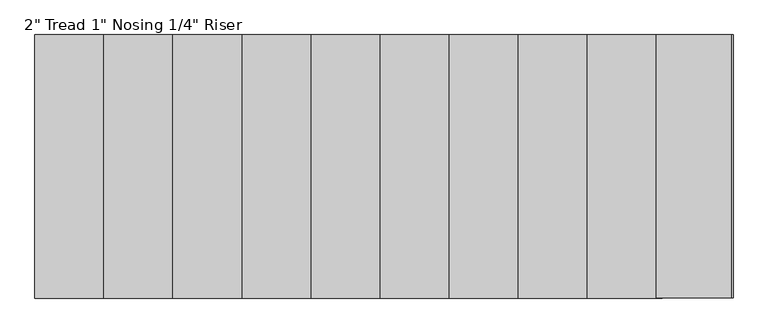
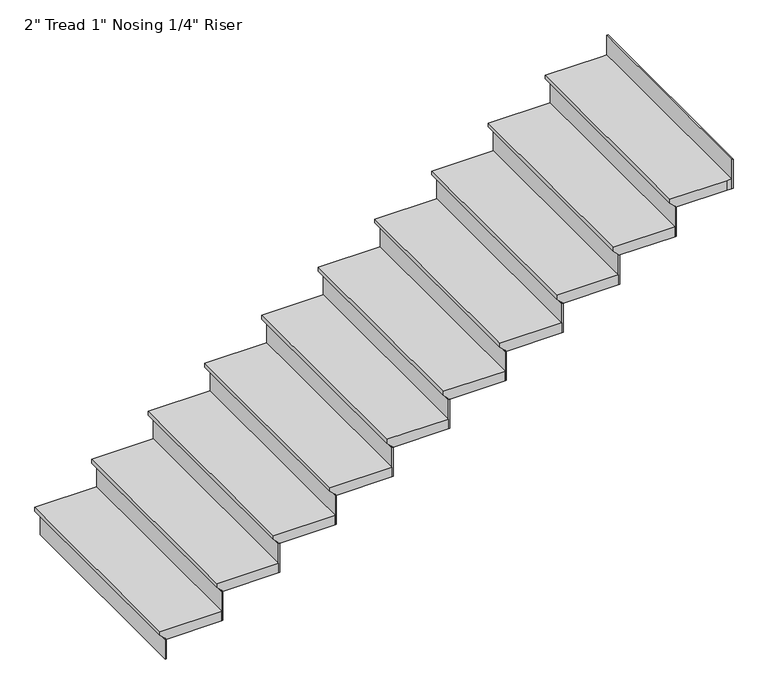
"""IFC4 building model written with IfcOpenShell, lengths in millimetres: stair flight geometry."""

from ifc_helpers import new_model, si_unit, origin, place, context, project, spatial, faceted_brep, source, transform, mapped, element, save


def stair_flight_b15b2b3c(model_context):
    return source(origin(), model_context, "Body", "Brep", [
        faceted_brep([(-459.26646, -1849.1834702, 6229.35), (-459.26646, -1849.1834702, 6248.4), (-459.26646, -782.3834702, 6248.4), (-459.26646, -782.3834702, 6229.35), (-433.86646, -1849.1834702, 6203.95), (-433.86646, -782.3834702, 6203.95), (-154.46646, -1849.1834702, 6248.4), (-154.46646, -782.3834702, 6248.4), (-433.86646, -782.3834702, 6197.6), (-154.46646, -782.3834702, 6197.6), (-154.46646, -1849.1834702, 6197.6), (-433.86646, -1849.1834702, 6197.6)], [[[0, 1, 2, 3]], [[4, 0, 3, 5]], [[2, 1, 6, 7]], [[8, 9, 10, 11]], [[2, 7, 9, 8, 5, 3]], [[8, 11, 4, 5]], [[6, 1, 0, 4, 11, 10]], [[7, 6, 10, 9]]]),
        faceted_brep([(-433.86646, -1849.1834702, 6197.6), (-433.86646, -1849.1834702, 6096.0), (-427.51646, -1849.1834702, 6096.0), (-427.51646, -1849.1834702, 6197.6), (-433.86646, -782.3834702, 6197.6), (-427.51646, -782.3834702, 6197.6), (-427.51646, -782.3834702, 6096.0), (-433.86646, -782.3834702, 6096.0)], [[[0, 1, 2, 3]], [[4, 5, 6, 7]], [[1, 0, 4, 7]], [[2, 1, 7, 6]], [[3, 2, 6, 5]], [[0, 3, 5, 4]]]),
        faceted_brep([(-154.46646, -1849.1834702, 6350.0), (-154.46646, -1849.1834702, 6197.6), (-148.11646, -1849.1834702, 6197.6), (-148.11646, -1849.1834702, 6350.0), (-154.46646, -782.3834702, 6350.0), (-148.11646, -782.3834702, 6350.0), (-148.11646, -782.3834702, 6197.6), (-154.46646, -782.3834702, 6197.6)], [[[0, 1, 2, 3]], [[4, 5, 6, 7]], [[1, 0, 4, 7]], [[2, 1, 7, 6]], [[3, 2, 6, 5]], [[0, 3, 5, 4]]]),
        faceted_brep([(-179.86646, -782.3834702, 6400.8), (-179.86646, -1849.1834702, 6400.8), (124.93354, -1849.1834702, 6400.8), (124.93354, -782.3834702, 6400.8), (-154.46646, -782.3834702, 6350.0), (124.93354, -782.3834702, 6350.0), (124.93354, -1849.1834702, 6350.0), (-154.46646, -1849.1834702, 6350.0), (-154.46646, -782.3834702, 6356.35), (-179.86646, -782.3834702, 6381.75), (-154.46646, -1849.1834702, 6356.35), (-179.86646, -1849.1834702, 6381.75)], [[[0, 1, 2, 3]], [[4, 5, 6, 7]], [[0, 3, 5, 4, 8, 9]], [[4, 7, 10, 8]], [[2, 1, 11, 10, 7, 6]], [[3, 2, 6, 5]], [[11, 1, 0, 9]], [[10, 11, 9, 8]]]),
        faceted_brep([(124.93354, -1849.1834702, 6502.4), (124.93354, -1849.1834702, 6350.0), (131.28354, -1849.1834702, 6350.0), (131.28354, -1849.1834702, 6502.4), (124.93354, -782.3834702, 6502.4), (131.28354, -782.3834702, 6502.4), (131.28354, -782.3834702, 6350.0), (124.93354, -782.3834702, 6350.0)], [[[0, 1, 2, 3]], [[4, 5, 6, 7]], [[1, 0, 4, 7]], [[2, 1, 7, 6]], [[3, 2, 6, 5]], [[0, 3, 5, 4]]]),
        faceted_brep([(99.53354, -782.3834702, 6553.2), (99.53354, -1849.1834702, 6553.2), (404.33354, -1849.1834702, 6553.2), (404.33354, -782.3834702, 6553.2), (124.93354, -782.3834702, 6502.4), (404.33354, -782.3834702, 6502.4), (404.33354, -1849.1834702, 6502.4), (124.93354, -1849.1834702, 6502.4), (124.93354, -782.3834702, 6508.75), (99.53354, -782.3834702, 6534.15), (124.93354, -1849.1834702, 6508.75), (99.53354, -1849.1834702, 6534.15)], [[[0, 1, 2, 3]], [[4, 5, 6, 7]], [[0, 3, 5, 4, 8, 9]], [[4, 7, 10, 8]], [[2, 1, 11, 10, 7, 6]], [[3, 2, 6, 5]], [[11, 1, 0, 9]], [[10, 11, 9, 8]]]),
        faceted_brep([(404.33354, -1849.1834702, 6654.8), (404.33354, -1849.1834702, 6502.4), (410.68354, -1849.1834702, 6502.4), (410.68354, -1849.1834702, 6654.8), (404.33354, -782.3834702, 6654.8), (410.68354, -782.3834702, 6654.8), (410.68354, -782.3834702, 6502.4), (404.33354, -782.3834702, 6502.4)], [[[0, 1, 2, 3]], [[4, 5, 6, 7]], [[1, 0, 4, 7]], [[2, 1, 7, 6]], [[3, 2, 6, 5]], [[0, 3, 5, 4]]]),
        faceted_brep([(378.93354, -782.3834702, 6705.6), (378.93354, -1849.1834702, 6705.6), (683.73354, -1849.1834702, 6705.6), (683.73354, -782.3834702, 6705.6), (404.33354, -782.3834702, 6654.8), (683.73354, -782.3834702, 6654.8), (683.73354, -1849.1834702, 6654.8), (404.33354, -1849.1834702, 6654.8), (404.33354, -782.3834702, 6661.15), (378.93354, -782.3834702, 6686.55), (404.33354, -1849.1834702, 6661.15), (378.93354, -1849.1834702, 6686.55)], [[[0, 1, 2, 3]], [[4, 5, 6, 7]], [[0, 3, 5, 4, 8, 9]], [[4, 7, 10, 8]], [[2, 1, 11, 10, 7, 6]], [[3, 2, 6, 5]], [[11, 1, 0, 9]], [[10, 11, 9, 8]]]),
        faceted_brep([(683.73354, -1849.1834702, 6807.2), (683.73354, -1849.1834702, 6654.8), (690.08354, -1849.1834702, 6654.8), (690.08354, -1849.1834702, 6807.2), (683.73354, -782.3834702, 6807.2), (690.08354, -782.3834702, 6807.2), (690.08354, -782.3834702, 6654.8), (683.73354, -782.3834702, 6654.8)], [[[0, 1, 2, 3]], [[4, 5, 6, 7]], [[1, 0, 4, 7]], [[2, 1, 7, 6]], [[3, 2, 6, 5]], [[0, 3, 5, 4]]]),
        faceted_brep([(658.33354, -782.3834702, 6858.0), (658.33354, -1849.1834702, 6858.0), (963.13354, -1849.1834702, 6858.0), (963.13354, -782.3834702, 6858.0), (683.73354, -782.3834702, 6807.2), (963.13354, -782.3834702, 6807.2), (963.13354, -1849.1834702, 6807.2), (683.73354, -1849.1834702, 6807.2), (683.73354, -782.3834702, 6813.55), (658.33354, -782.3834702, 6838.95), (683.73354, -1849.1834702, 6813.55), (658.33354, -1849.1834702, 6838.95)], [[[0, 1, 2, 3]], [[4, 5, 6, 7]], [[0, 3, 5, 4, 8, 9]], [[4, 7, 10, 8]], [[2, 1, 11, 10, 7, 6]], [[3, 2, 6, 5]], [[11, 1, 0, 9]], [[10, 11, 9, 8]]]),
        faceted_brep([(963.13354, -1849.1834702, 6959.6), (963.13354, -1849.1834702, 6807.2), (969.48354, -1849.1834702, 6807.2), (969.48354, -1849.1834702, 6959.6), (963.13354, -782.3834702, 6959.6), (969.48354, -782.3834702, 6959.6), (969.48354, -782.3834702, 6807.2), (963.13354, -782.3834702, 6807.2)], [[[0, 1, 2, 3]], [[4, 5, 6, 7]], [[1, 0, 4, 7]], [[2, 1, 7, 6]], [[3, 2, 6, 5]], [[0, 3, 5, 4]]]),
        faceted_brep([(937.73354, -782.3834702, 7010.4), (937.73354, -1849.1834702, 7010.4), (1242.53354, -1849.1834702, 7010.4), (1242.53354, -782.3834702, 7010.4), (963.13354, -782.3834702, 6959.6), (1242.53354, -782.3834702, 6959.6), (1242.53354, -1849.1834702, 6959.6), (963.13354, -1849.1834702, 6959.6), (963.13354, -782.3834702, 6965.95), (937.73354, -782.3834702, 6991.35), (963.13354, -1849.1834702, 6965.95), (937.73354, -1849.1834702, 6991.35)], [[[0, 1, 2, 3]], [[4, 5, 6, 7]], [[0, 3, 5, 4, 8, 9]], [[4, 7, 10, 8]], [[2, 1, 11, 10, 7, 6]], [[3, 2, 6, 5]], [[11, 1, 0, 9]], [[10, 11, 9, 8]]]),
        faceted_brep([(1242.53354, -1849.1834702, 7112.0), (1242.53354, -1849.1834702, 6959.6), (1248.88354, -1849.1834702, 6959.6), (1248.88354, -1849.1834702, 7112.0), (1242.53354, -782.3834702, 7112.0), (1248.88354, -782.3834702, 7112.0), (1248.88354, -782.3834702, 6959.6), (1242.53354, -782.3834702, 6959.6)], [[[0, 1, 2, 3]], [[4, 5, 6, 7]], [[1, 0, 4, 7]], [[2, 1, 7, 6]], [[3, 2, 6, 5]], [[0, 3, 5, 4]]]),
        faceted_brep([(1217.13354, -782.3834702, 7162.8), (1217.13354, -1849.1834702, 7162.8), (1521.93354, -1849.1834702, 7162.8), (1521.93354, -782.3834702, 7162.8), (1242.53354, -782.3834702, 7112.0), (1521.93354, -782.3834702, 7112.0), (1521.93354, -1849.1834702, 7112.0), (1242.53354, -1849.1834702, 7112.0), (1242.53354, -782.3834702, 7118.35), (1217.13354, -782.3834702, 7143.75), (1242.53354, -1849.1834702, 7118.35), (1217.13354, -1849.1834702, 7143.75)], [[[0, 1, 2, 3]], [[4, 5, 6, 7]], [[0, 3, 5, 4, 8, 9]], [[4, 7, 10, 8]], [[2, 1, 11, 10, 7, 6]], [[3, 2, 6, 5]], [[11, 1, 0, 9]], [[10, 11, 9, 8]]]),
        faceted_brep([(1521.93354, -1849.1834702, 7264.4), (1521.93354, -1849.1834702, 7112.0), (1528.28354, -1849.1834702, 7112.0), (1528.28354, -1849.1834702, 7264.4), (1521.93354, -782.3834702, 7264.4), (1528.28354, -782.3834702, 7264.4), (1528.28354, -782.3834702, 7112.0), (1521.93354, -782.3834702, 7112.0)], [[[0, 1, 2, 3]], [[4, 5, 6, 7]], [[1, 0, 4, 7]], [[2, 1, 7, 6]], [[3, 2, 6, 5]], [[0, 3, 5, 4]]]),
        faceted_brep([(1496.53354, -782.3834702, 7315.2), (1496.53354, -1849.1834702, 7315.2), (1801.33354, -1849.1834702, 7315.2), (1801.33354, -782.3834702, 7315.2), (1521.93354, -782.3834702, 7264.4), (1801.33354, -782.3834702, 7264.4), (1801.33354, -1849.1834702, 7264.4), (1521.93354, -1849.1834702, 7264.4), (1521.93354, -782.3834702, 7270.75), (1496.53354, -782.3834702, 7296.15), (1521.93354, -1849.1834702, 7270.75), (1496.53354, -1849.1834702, 7296.15)], [[[0, 1, 2, 3]], [[4, 5, 6, 7]], [[0, 3, 5, 4, 8, 9]], [[4, 7, 10, 8]], [[2, 1, 11, 10, 7, 6]], [[3, 2, 6, 5]], [[11, 1, 0, 9]], [[10, 11, 9, 8]]]),
        faceted_brep([(1801.33354, -1849.1834702, 7416.8), (1801.33354, -1849.1834702, 7264.4), (1807.68354, -1849.1834702, 7264.4), (1807.68354, -1849.1834702, 7416.8), (1801.33354, -782.3834702, 7416.8), (1807.68354, -782.3834702, 7416.8), (1807.68354, -782.3834702, 7264.4), (1801.33354, -782.3834702, 7264.4)], [[[0, 1, 2, 3]], [[4, 5, 6, 7]], [[1, 0, 4, 7]], [[2, 1, 7, 6]], [[3, 2, 6, 5]], [[0, 3, 5, 4]]]),
        faceted_brep([(1775.93354, -782.3834702, 7467.6), (1775.93354, -1849.1834702, 7467.6), (2080.73354, -1849.1834702, 7467.6), (2080.73354, -782.3834702, 7467.6), (1801.33354, -782.3834702, 7416.8), (2080.73354, -782.3834702, 7416.8), (2080.73354, -1849.1834702, 7416.8), (1801.33354, -1849.1834702, 7416.8), (1801.33354, -782.3834702, 7423.15), (1775.93354, -782.3834702, 7448.55), (1801.33354, -1849.1834702, 7423.15), (1775.93354, -1849.1834702, 7448.55)], [[[0, 1, 2, 3]], [[4, 5, 6, 7]], [[0, 3, 5, 4, 8, 9]], [[4, 7, 10, 8]], [[2, 1, 11, 10, 7, 6]], [[3, 2, 6, 5]], [[11, 1, 0, 9]], [[10, 11, 9, 8]]]),
        faceted_brep([(2360.13354, -1849.1834702, 7721.6), (2360.13354, -1849.1834702, 7569.2), (2366.48354, -1849.1834702, 7569.2), (2366.48354, -1849.1834702, 7721.6), (2360.13354, -782.3834702, 7721.6), (2366.48354, -782.3834702, 7721.6), (2366.48354, -782.3834702, 7569.2), (2360.13354, -782.3834702, 7569.2)], [[[0, 1, 2, 3]], [[4, 5, 6, 7]], [[1, 0, 4, 7]], [[2, 1, 7, 6]], [[3, 2, 6, 5]], [[0, 3, 5, 4]]]),
        faceted_brep([(2080.73354, -1849.1834702, 7569.2), (2080.73354, -1849.1834702, 7416.8), (2087.08354, -1849.1834702, 7416.8), (2087.08354, -1849.1834702, 7569.2), (2080.73354, -782.3834702, 7569.2), (2087.08354, -782.3834702, 7569.2), (2087.08354, -782.3834702, 7416.8), (2080.73354, -782.3834702, 7416.8)], [[[0, 1, 2, 3]], [[4, 5, 6, 7]], [[1, 0, 4, 7]], [[2, 1, 7, 6]], [[3, 2, 6, 5]], [[0, 3, 5, 4]]]),
        faceted_brep([(2360.13354, -782.3834702, 7620.0), (2334.73354, -782.3834702, 7620.0), (2055.33354, -782.3834702, 7620.0), (2055.33354, -1849.1834702, 7620.0), (2334.73354, -1849.1834702, 7620.0), (2360.13354, -1849.1834702, 7620.0), (2334.73354, -782.3834702, 7569.2), (2360.13354, -782.3834702, 7569.2), (2360.13354, -1849.1834702, 7569.2), (2334.73354, -1849.1834702, 7569.2), (2080.73354, -1849.1834702, 7569.2), (2080.73354, -782.3834702, 7569.2), (2080.73354, -782.3834702, 7575.55), (2055.33354, -782.3834702, 7600.95), (2080.73354, -1849.1834702, 7575.55), (2055.33354, -1849.1834702, 7600.95)], [[[0, 1, 2, 3, 4, 5]], [[6, 7, 8, 9, 10, 11]], [[1, 0, 7, 6]], [[2, 1, 6, 11, 12, 13]], [[11, 10, 14, 12]], [[4, 3, 15, 14, 10, 9]], [[5, 4, 9, 8]], [[0, 5, 8, 7]], [[15, 3, 2, 13]], [[14, 15, 13, 12]]]),
    ])


if __name__ == "__main__":
    model = new_model("IFC4")
    model_context = context("Model", 3, world=origin())
    ifc_project = project(units=[si_unit("LENGTHUNIT", "METRE", prefix="MILLI")], contexts=[model_context])
    site = spatial("IfcSite", under=ifc_project)
    building = spatial("IfcBuilding", under=site)
    placement = place(None, origin())
    stair_flight_shape = stair_flight_b15b2b3c(model_context)
    element("IfcStairFlight", 1, ObjectType="2\" Tread 1\" Nosing 1/4\" Riser", at=placement, inside=building, context=model_context, shape_type="MappedRepresentation", body=[
        mapped(stair_flight_shape, transform((0.0, 0.0, 0.0), x_axis=(1.0, 0.0, 0.0), y_axis=(0.0, 1.0, 0.0), z_axis=(0.0, 0.0, 1.0))),
    ])
    save(model, "model.ifc")
